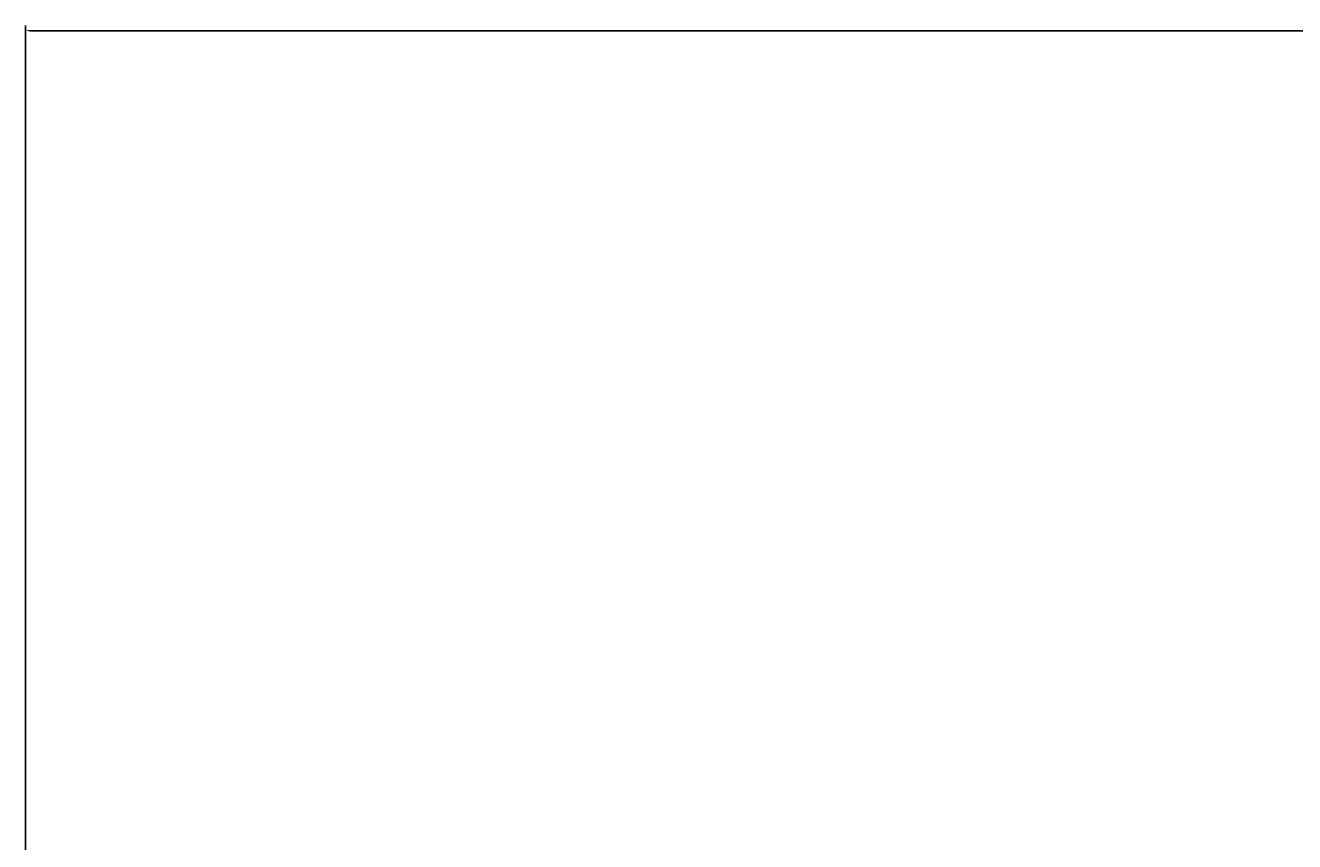
# Model space of a CAD drawing. Units: inches. Extents: x 7359 to 7979, y 33027 to 34263.
# Tile 19 of 32: x 7469 to 7511, y 33630 to 33657. Entities that reach past the tile are written whole.
import ezdxf

# ---------------------------------------------------------------- set-up
doc = ezdxf.new("R2010")
doc.units = ezdxf.units.IN
doc.layers.add('A-ANNO-DIMS', color=2, linetype='Continuous', lineweight=18)
doc.styles.get("Standard").update_dxf_attribs({"font": 'arial.ttf'})
doc.dimstyles.get("Standard").update_dxf_attribs({"dimtxt": 0.18, "dimasz": 0.18, "dimexe": 0.18, "dimexo": 0.0625, "dimgap": 0.09, "dimtad": 0, "dimtih": 1, "dimtoh": 1, "dimdec": 4, "dimzin": 0, "dimdsep": 46, "dimtxsty": 'Standard', "dimcen": 0.09, "dimadec": 0, "dimazin": 0, "dimtfac": 1, "dimtdec": 4, "dimtofl": 0, "dimtmove": 0, "dimatfit": 3, "dimfxl": 1, "dimtolj": 1, "dimtzin": 0, "dimarcsym": 0})

# ---------------------------------------------------------------- blocks, each defined once
blk = doc.blocks.new('*D66')
at = {"layer": 'A-ANNO-DIMS', "color": 0, "lineweight": -2, "transparency": 16777216}
for p, q in [((7468.727, 33627.225), (7468.727, 33657.242)), ((7468.907, 33657.062), (7681.03, 33657.062)), ((7893.947, 33657.062), (7681.824, 33657.062)), ((7894.127, 33627.225), (7894.127, 33657.242))]:
    blk.add_line(p, q, dxfattribs=at)
at = {"layer": 'A-ANNO-DIMS', "color": 0, "transparency": 16777216}
for points in [[(7468.907, 33657.092), (7468.907, 33657.032), (7468.727, 33657.062)], [(7893.947, 33657.092), (7893.947, 33657.032), (7894.127, 33657.062)]]:
    blk.add_solid(points, dxfattribs=at)
at = {"layer": 'Defpoints', "color": 0, "transparency": 16777216}
for p in [(7894.127, 33657.062), (7468.727, 33627.162), (7894.127, 33627.162)]:
    blk.add_point(p, dxfattribs=at)
at = {"layer": 'A-ANNO-DIMS', "color": 0, "transparency": 16777216, "insert": (7681.427, 33657.062), "char_height": 0.18, "attachment_point": 5}
blk.add_mtext('\\A1;425.4', dxfattribs=at)

msp = doc.modelspace()

# ---------------------------------------------------------------- dimensions: what is measured, and where the dimension line sits
at = {"layer": 'A-ANNO-DIMS'}
dim = msp.add_linear_dim(base=(7894.1266, 33657.0623), p1=(7468.7266, 33627.1623), p2=(7894.1266, 33627.1623), dimstyle='Standard', override={"dimdec": 1, "dimlfac": 1, "dimrnd": 0, "dimzin": 0, "dimdsep": 46, "dimlunit": 2}, dxfattribs=at)
dim.commit()
dim.dimension.update_dxf_attribs({"geometry": '*D66', "text_midpoint": (7681.4266, 33657.0623)})

doc.saveas('drawing.dxf')
